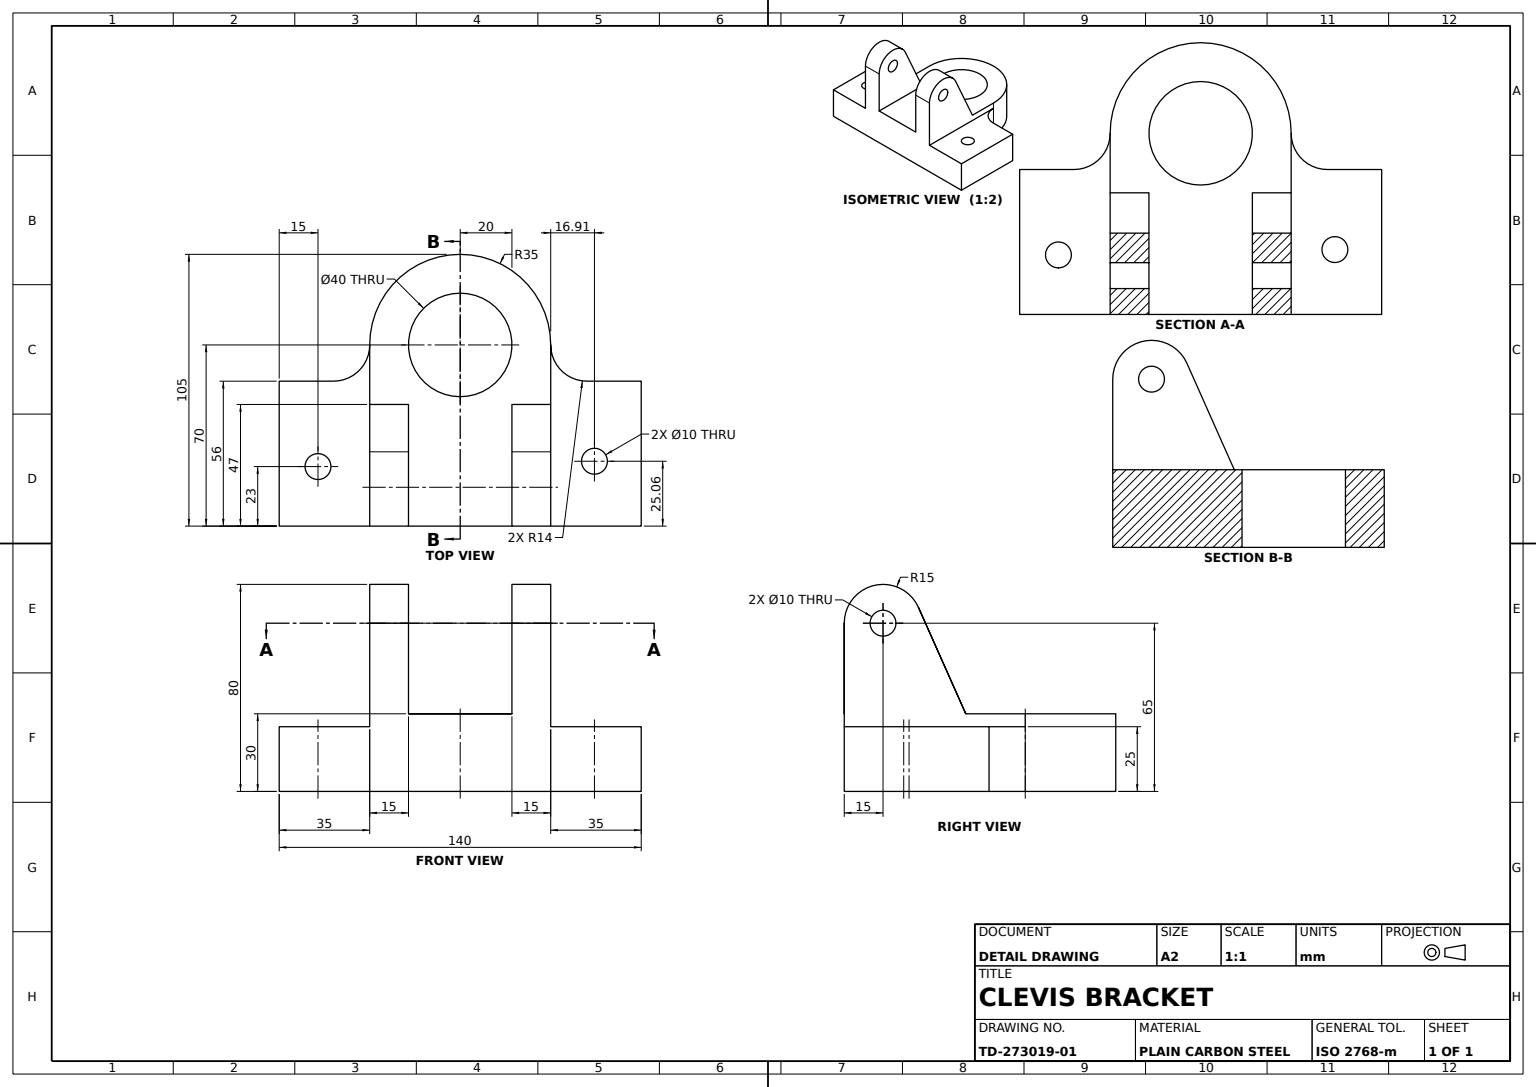
SolidWorks part; units mm, degrees
material "Plain Carbon Steel"
ref_plane "Front Plane" through (0, 0, 0) normal (0, 0, 1) x (1, 0, 0)
ref_plane "Top Plane" through (0, 0, 0) normal (0, 1, 0) x (1, 0, 0)
ref_plane "Right Plane" through (0, 0, 0) normal (1, 0, 0) x (0, 0, -1)
sketch "Base Plate Sketch" plane through (0, 0, 0) normal (0, 1, 0) x (1, 0, 0)
  line L0 (-70, 95.1003) -> (70, 95.1003)
  line L1 (-70, 73.2698) -> (-70, -31.7302)
  line L2 (70, 73.2698) -> (70, -31.7302)
  line L3 (-70, 73.2698) -> (-70, 95.1003)
  line L4 (70, 73.2698) -> (70, 95.1003)
  line L5 (-70, -31.7302) -> (70, -31.7302)
  dimension "D1" = 70
  dimension "D2" = 105
  dimension "D7" = 140
  dimension "D3" = 21.8306
  dimension "D4" = 31.7302
extrude "Base Plate" add sketch "Base Plate Sketch" along normal blind 25
sketch "Housing Profile Cut Sketch" plane through (0, 25, 0) normal (0, 1, 0) x (1, 0, 0)
  line L0 (70, -31.7302) -> (70, 24.2698)
  line L1 (70, -31.7302) -> (70, 95.1003) construction
  line L2 (70, 24.2698) -> (49, 24.2698)
  line L3 (-70, 95.1003) -> (-70, -31.7302) construction
  line L4 (-70, 24.2698) -> (-70, -31.7302)
  line L5 (-49, 24.2698) -> (-70, 24.2698)
  line L7 (-70, 95.1003) -> (70, 95.1003)
  line L8 (-70, 95.1003) -> (-70, -31.7302)
  line L9 (-70, -31.7302) -> (70, -31.7302)
  line L10 (70, 95.1003) -> (70, -31.7302)
  arc A0 (35, 38.2698) -> (-35, 38.2698) centre (0, 38.2698) ccw
  arc A1 (35, 38.2698) -> (49, 24.2698) centre (49, 38.2698) ccw
  arc A2 (-49, 24.2698) -> (-35, 38.2698) centre (-49, 38.2698) ccw
  dimension "D1" = 70
  dimension "D4" = 14
  dimension "D5" = 14
  dimension "D2" = 70
  dimension "D3" = 56
extrude "Housing Profile Cut" cut sketch "Housing Profile Cut Sketch" against normal blind 91 and the other way blind 61 contours L5 A2 A0 A1 L2 L1 L3
sketch "Housing Reference Sketch" plane through (0, 25, 0) normal (0, 1, 0) x (1, 0, 0)
  circle A0 centre (0, 38.2698) radius 35
  dimension "D1" = 70
sketch "Housing Boss Sketch" plane through (0, 25, 0) normal (0, 1, 0) x (1, 0, 0)
  line L0 (35, 38.2698) -> (35, -31.7302)
  line L1 (-70, -31.7302) -> (70, -31.7302) construction
  line L2 (-35, 38.2698) -> (-35, -31.7302)
  line L3 (-35, -31.7302) -> (35, -31.7302)
  circle A0 centre (0, 38.2698) radius 35
  line M4 (-70, -31.7302) -> (70, -31.7302)
  arc M8 (35, 38.2698) -> (-35, 38.2698) centre (0, 38.2698) ccw
extrude "Housing Boss" add sketch "Housing Boss Sketch" along normal blind 5 contours A0 M8 | A0 L2 L0 M4
sketch "Bore Ø40 Sketch" plane through (0, 30, 0) normal (0, 1, 0) x (1, 0, 0)
  circle A0 centre (0, 38.2698) radius 20
  dimension "D1" = 40
extrude "Bore Ø40" cut sketch "Bore Ø40 Sketch" against normal blind 116 and the other way blind 110
sketch "Mounting Hole Ø10 A Sketch" plane through (0, 25, 0) normal (0, 1, 0) x (1, 0, 0)
  line L0 (-70, 24.2698) -> (-70, -31.7302) construction
  circle A0 centre (-55, -8.7302) radius 5
  dimension "D1" = 10
  dimension "D2" = 23
  dimension "D3" = 15
extrude "Mounting Hole Ø10 A" cut sketch "Mounting Hole Ø10 A Sketch" against normal blind 393
sketch "Mounting Hole Ø10 B Sketch" plane through (0, 25, 0) normal (0, 1, 0) x (1, 0, 0)
  line L0 (35, 38.2698) -> (35, -31.7302) construction
  circle A0 centre (51.914, -6.6665) radius 5
  dimension "D1" = 10
  dimension "D2" = 16.914
  dimension "D3" = 25.0638
extrude "Mounting Hole Ø10 B" cut sketch "Mounting Hole Ø10 B Sketch" against normal blind 393 and the other way blind 393
sketch "Clevis Lugs Sketch" plane through (35, 0, 0) normal (1, 0, 0) x (0, 0, -1)
  line L0 (-31.7302, 30) -> (-31.7302, 65)
  line L2 (-31.7302, 30) -> (15.2698, 30)
  line L3 (15.2698, 30) -> (-3.4909, 72.1429)
  arc A0 (-3.0267, 71.1003) -> (-31.7302, 65) centre (-16.7302, 65) ccw
  line M6 (38.2698, 30) -> (-31.7302, 30)
  dimension "D4" = 41.7606
  dimension "D2" = 15
  dimension "D1" = 65
  dimension "D3" = 47
extrude "Clevis Lugs" add sketch "Clevis Lugs Sketch" against normal blind 70 contours L3 A0 L0 M6
sketch "Lug Gap Cut Sketch" plane through (0, 30, 0) normal (0, 1, 0) x (1, 0, 0)
  line L0 (-20, 15.2698) -> (-20, -31.7302)
  line L1 (20, 15.2698) -> (20, -31.7302)
  line L2 (-20, 15.2698) -> (20, 15.2698)
  line L4 (-20, -31.7302) -> (20, -31.7302)
  dimension "D1" = 15
  dimension "D2" = 40
  dimension "D3" = 47
  dimension "D4" = 31.7302
extrude "Lug Gap Cut" cut sketch "Lug Gap Cut Sketch" along normal blind 207
sketch "Pin Hole Ø10 Sketch" plane through (-35, 0, 0) normal (-1, 0, 0) x (0, 0, 1)
  circle A0 centre (16.7302, 65) radius 5
  dimension "D1" = 10
extrude "Pin Hole Ø10" cut sketch "Pin Hole Ø10 Sketch" against normal blind 207 and the other way blind 207
